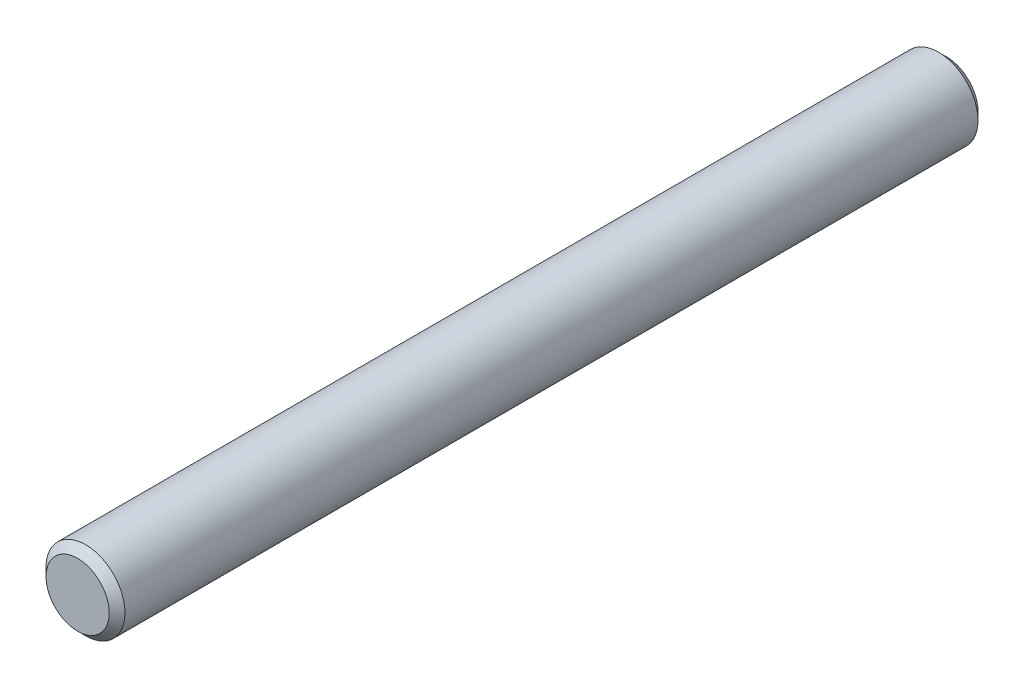
from build123d import *

# Parameters (mm, degrees)
PIN_PROFILE_5_R          = 2.5
PIN_BODY_5X55_DEPTH      = 27.5
END_CHAMFERS_0_5X45_SIZE = 0.5


with BuildPart() as part:
    # Pin Profile Ø5 → Pin Body Ø5x55 (new, symmetric)
    with BuildSketch(Plane.XY):
        Circle(PIN_PROFILE_5_R)
    extrude(amount=PIN_BODY_5X55_DEPTH, both=True)

    # End Chamfers 0.5x45°
    end_chamfers_0_5x45_edges = [part.edges().sort_by_distance(p)[0] for p in [
        (-2.5, 0, -27.5),
        (-2.5, 0, 27.5),
    ]]
    chamfer(end_chamfers_0_5x45_edges, length=END_CHAMFERS_0_5X45_SIZE)


solid = part.part
